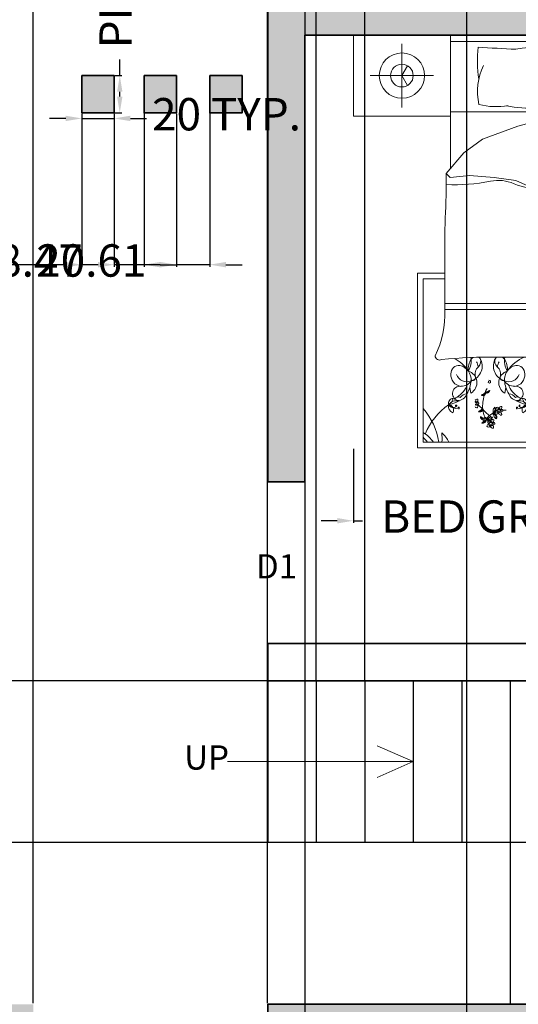
# Model space of a CAD drawing. Units: centimetres. Extents: x 2137 to 3697, y 183 to 2094.
# Tile 5 of 8: x 3031 to 3339, y 600 to 1208. Entities that reach past the tile are written whole.
import ezdxf

# ---------------------------------------------------------------- set-up
doc = ezdxf.new("R2010")
doc.units = ezdxf.units.CM
for name, color, linetype, lineweight in [('A-ANNO-DIMS', 2, 'Continuous', 18), ('A-ANNO-SYMB', 7, 'Continuous', 18), ('A-ANNO-TEXT', 7, 'Continuous', 18), ('A-COLS', 7, 'Continuous', 35), ('A-COLS-PATT', 52, 'Continuous', 13), ('A-FLOR-STRS', 7, 'Continuous', 25), ('A-FURN', 8, 'Continuous', 18), ('A-WALL', 7, 'Continuous', 35), ('A-WALL-PATT', 52, 'Continuous', 13)]:
    doc.layers.add(name, color=color, linetype=linetype, lineweight=lineweight)
doc.styles.get("Standard").update_dxf_attribs({"font": 'arial.ttf'})
doc.dimstyles.new('ISO-25', dxfattribs={"dimtxt": 20, "dimasz": 10, "dimexe": 1.25, "dimexo": 0.625, "dimtad": 0, "dimtxsty": 'Standard', "dimcen": 2.5, "dimadec": 0, "dimazin": 0, "dimtfac": 1, "dimtmove": 0, "dimatfit": 3, "dimfxl": 1, "dimarcsym": 0})

# ---------------------------------------------------------------- blocks, each defined once
blk = doc.blocks.new('BED')
for p, q in [((2442.52, 2474.71), (2742.52, 2474.71)), ((2502.52, 2474.71), (2502.52, 2392.37)), ((2682.52, 2470.86), (2502.52, 2470.86)), ((2472.52, 2430.11), (2472.52, 2469.31)), ((2712.52, 2430.11), (2712.52, 2469.31)), ((2492.12, 2449.71), (2452.92, 2449.71)), ((2692.92, 2449.71), (2732.12, 2449.71)), ((2502.52, 2427.3), (2682.52, 2427.3)), ((2544.19, 2418.38), (2576.9, 2427.3)), ((2584.93, 2427.3), (2568.49, 2404.42)), ((2522.31, 2410.49), (2544.19, 2418.38)), ((2510.77, 2401.99), (2522.31, 2410.49)), ((2681.6, 2411.76), (2572.66, 2410.22)), ((2681.71, 2414.84), (2574.9, 2413.34)), ((2568.49, 2404.42), (2561.81, 2386.81)), ((2499.83, 2389.24), (2510.77, 2401.99)), ((2681.46, 2399.23), (2566.35, 2398.76)), ((2681.44, 2402.31), (2567.52, 2401.86)), ((2502.26, 2386.81), (2499.83, 2389.24)), ((2514.41, 2388.02), (2502.26, 2386.81)), ((2529.61, 2386.81), (2514.41, 2388.02)), ((2542.97, 2384.99), (2529.61, 2386.81)), ((2561.81, 2386.81), (2560.59, 2378.91)), ((2550.87, 2381.34), (2542.97, 2384.99)), ((2560.59, 2378.91), (2550.87, 2381.34)), ((2482.11, 2327.65), (2499.08, 2327.65)), ((2482.11, 2219.58), (2482.11, 2327.65)), ((2684.19, 2327.65), (2700.83, 2327.65)), ((2700.83, 2327.65), (2700.83, 2219.58)), ((2499.08, 2324.17), (2485.59, 2324.17)), ((2485.59, 2324.17), (2485.59, 2223.06)), ((2697.35, 2324.17), (2684.13, 2324.17)), ((2697.35, 2223.06), (2697.35, 2324.17)), ((2683.88, 2308.94), (2499.06, 2308.94)), ((2684.17, 2305.2), (2499.06, 2305.2)), ((2653.42, 2275.73), (2531.62, 2275.73)), ((2515.15, 2253.47), (2514.49, 2256.86)), ((2536.12, 2253.47), (2536.78, 2256.86)), ((2646.82, 2253.47), (2646.16, 2256.86)), ((2667.79, 2253.47), (2668.45, 2256.86)), ((2485.59, 2223.06), (2697.35, 2223.06)), ((2700.83, 2219.58), (2482.11, 2219.58))]:
    blk.add_line(p, q)
for points in [[(2502.52, 2424.71), (2442.52, 2424.71), (2442.52, 2474.71)], [(2682.52, 2474.71), (2682.52, 2424.71), (2742.52, 2424.71), (2742.52, 2474.71)], [(2472.52, 2449.71), (2476.02, 2455.77)], [(2712.52, 2449.71), (2709.02, 2455.77)], [(2472.52, 2449.71), (2476.02, 2443.65)], [(2712.52, 2449.71), (2709.02, 2443.65)]]:
    blk.add_lwpolyline(points)
for points in [[(2519.75, 2467.23, 0.074897), (2520.11, 2447.64, -0.472817)], [(2591.11, 2446.54, 0.14099), (2591.71, 2466.53, 0.235245)], [(2603.92, 2446.54, -0.14099), (2603.32, 2466.53, -0.235245)], [(2665.29, 2467.23, -0.074897), (2664.92, 2447.64, 0.472817)], [(2499.2, 2361.77, 0.001242), (2499.06, 2304.85, -0.127202), (2493.05, 2276.48)], [(2683.8, 2311.3, 0.056112), (2685.97, 2294.79, 0.095341), (2690.19, 2278.9)]]:
    blk.add_lwpolyline(points, format="xyb")
for centre, radius in [((2472.52, 2449.71), 14), ((2712.52, 2449.71), 14), ((2472.52, 2449.71), 7), ((2712.52, 2449.71), 7), ((2532.49, 2242.6), 0.764), ((2650.46, 2242.6), 0.764), ((2527.49, 2234.55), 0.764), ((2655.45, 2234.55), 0.764)]:
    blk.add_circle(centre, radius)
for centre, radius, start, end in [((2685.11, 5322.24), 2859.79, 266.68521, 267.14978), ((2560.85, 2358.67), 108.8, 82.21958, 99.49698), ((2583.83, 2413.66), 53.46, 81.52493, 103.95996), ((2607.44, 2452.27), 14.84, 63.34374, 106.10256), ((2629.68, 2414.74), 52.74, 76.34271, 101.1841), ((2499.93, 5322.24), 2859.79, 272.85022, 273.31479), ((2557.97, 2439.77), 38.67, 155.1316, 191.75834), ((2627.07, 2439.77), 38.67, 348.24166, 24.8684), ((2555.75, 2436.51), 36.76, 354.01289, 15.82928), ((2639.29, 2436.51), 36.76, 164.17072, 185.98711), ((2530.45, 2470.74), 40.2, 255.10393, 281.03689), ((2551.61, 2499.32), 69.73, 258.03974, 289.26152), ((2579.84, 2484.1), 52.9, 259.86169, 283.62376), ((2609.45, 2447.1), 15.9, 245.01826, 288.54073), ((2637.23, 2467.78), 38.19, 243.87611, 286.17464), ((2654.58, 2470.74), 40.2, 258.96311, 284.89607), ((3220.32, 2390.64), 539.05, 176.09997, 180.92818), ((2224.76, 2381.78), 275.17, 355.82941, 1.55305), ((2504.97, 2495.47), 113.22, 267.45188, 281.3392), ((2532.03, 2360.52), 24.42, 66.26158, 101.3392), ((2581.42, 2492.28), 116.34, 250.11942, 259.33829), ((3384.42, 2371.04), 703.17, 179.11454, 184.87351), ((2559.91, 2378.67), 0.724, 268.86235, 19.75363), ((2495.81, 2276.67), 2.77, 183.97998, 297.34124), ((2687.92, 2277.37), 2.73, 246.52186, 33.82642), ((2528.04, 1963.45), 312.3, 89.34325, 95.68869), ((2507.86, 2265.5), 5.07, 84.48557, 181.05378), ((2494.64, 2254.6), 22.71, 33.66712, 63.29966), ((2506.31, 2261.76), 9.02, 355.29334, 76.921), ((2525.07, 2268.11), 11.57, 145.78505, 184.73037), ((2502.97, 2273.51), 12.43, 328.82178, 9.15542), ((2518.36, 2272.41), 3.61, 120.0293, 142.32497), ((2512.59, 2270.28), 9.56, 289.28218, 29.1751), ((2511.15, 2268.55), 8.62, 7.43599, 29.91487), ((2516.83, 2273.13), 4.49, 311.56531, 23.83541), ((2518.36, 2272.41), 3.61, 44.45169, 63.55801), ((2538.68, 2270.28), 9.56, 150.8249, 250.71782), ((2534.44, 2273.13), 4.49, 156.16459, 228.43469), ((2532.91, 2272.41), 3.61, 113.22901, 135.54831), ((2540.13, 2268.55), 8.62, 150.08513, 172.56401), ((2532.91, 2272.41), 3.61, 37.67503, 66.71436), ((2526.21, 2268.11), 11.57, 355.26963, 34.21495), ((2548.31, 2273.51), 12.43, 169.71335, 211.17822), ((2544.97, 2261.76), 9.02, 103.079, 184.70666), ((2556.64, 2254.6), 22.71, 111.49413, 146.33288), ((2543.41, 2265.5), 5.07, 358.94622, 95.51443), ((2639.53, 2265.5), 5.07, 84.48557, 181.05378), ((2626.3, 2254.6), 22.71, 33.66712, 68.50587), ((2637.98, 2261.76), 9.02, 355.29334, 76.921), ((2656.73, 2268.11), 11.57, 145.78505, 184.73037), ((2634.63, 2273.51), 12.43, 328.82178, 10.28665), ((2650.03, 2272.41), 3.61, 113.28564, 142.32497), ((2644.26, 2270.28), 9.56, 289.28218, 29.1751), ((2642.81, 2268.55), 8.62, 7.43599, 29.91487), ((2650.03, 2272.41), 3.61, 44.45169, 66.71436), ((2648.5, 2273.13), 4.49, 311.56531, 23.83541), ((2662.61, 1983.95), 291.92, 85.24024, 91.80351), ((2670.35, 2270.28), 9.56, 150.8249, 250.71782), ((2666.11, 2273.13), 4.49, 156.16459, 228.43469), ((2664.58, 2272.41), 3.61, 106.63434, 135.54831), ((2671.79, 2268.55), 8.62, 150.08513, 172.56401), ((2664.58, 2272.41), 3.61, 37.67503, 72.58143), ((2657.87, 2268.11), 11.57, 355.26963, 34.21495), ((2679.98, 2273.51), 12.43, 169.24899, 211.17822), ((2676.63, 2261.76), 9.02, 103.079, 184.70666), ((2688.3, 2254.6), 22.71, 113.64533, 146.33288), ((2675.08, 2265.5), 5.07, 358.94622, 95.51443), ((2509.94, 2264.78), 7.17, 174.94485, 262.88575), ((2512.76, 2267.5), 6.96, 201.58187, 291.42215), ((2511.44, 2259.94), 7.46, 299.90854, 73.1337), ((2523.89, 2265.16), 6.15, 131.56531, 195.14713), ((2527.38, 2265.16), 6.15, 344.85287, 48.43469), ((2539.84, 2259.94), 7.46, 106.8663, 240.09146), ((2538.52, 2267.5), 6.96, 248.57785, 338.41813), ((2541.33, 2264.78), 7.17, 277.11425, 5.05515), ((2641.61, 2264.78), 7.17, 174.94485, 262.88575), ((2644.43, 2267.5), 6.96, 201.58187, 291.42215), ((2643.1, 2259.94), 7.46, 299.90854, 73.1337), ((2655.56, 2265.16), 6.15, 131.56531, 195.14713), ((2659.05, 2265.16), 6.15, 344.85287, 48.43469), ((2671.51, 2259.94), 7.46, 106.8663, 240.09146), ((2670.18, 2267.5), 6.96, 248.57785, 338.41813), ((2673, 2264.78), 7.17, 277.11425, 5.05515), ((2499.37, 2263.14), 14.16, 301.26137, 341.7045), ((2508.7, 2266.37), 8.71, 272.3591, 324.04014), ((2499.23, 2262), 16.1, 326.28828, 356.5076), ((2525.07, 2268.11), 11.57, 212.70113, 216.34448), ((2516.16, 2263.07), 1.86, 257.30406, 15.14713), ((2526.5, 2260.25), 0.578, 102.70507, 280.43845), ((2526.43, 2260.6), 0.94, 280.43845, 100.41356), ((2535.12, 2263.07), 1.86, 164.85287, 282.69594), ((2526.21, 2268.11), 11.57, 323.65552, 327.29887), ((2542.58, 2266.37), 8.71, 215.95986, 267.6409), ((2552.04, 2262), 16.1, 183.4924, 213.71172), ((2551.91, 2263.14), 14.16, 198.2955, 238.73863), ((2594.92, 2255.93), 3.25, 63.02737, 163.80375), ((2591.63, 2263.52), 6.69, 271.45846, 315.37266), ((2598.02, 2255.93), 3.25, 16.19625, 116.97263), ((2601.31, 2263.52), 6.69, 224.62734, 268.54154), ((2631.03, 2263.14), 14.16, 301.26137, 341.7045), ((2640.36, 2266.37), 8.71, 272.3591, 324.04014), ((2630.9, 2262), 16.1, 326.28828, 356.5076), ((2656.73, 2268.11), 11.57, 212.70113, 216.34448), ((2647.82, 2263.07), 1.86, 257.30406, 15.14713), ((2656.51, 2260.6), 0.94, 79.58644, 259.56155), ((2656.44, 2260.25), 0.578, 259.56155, 77.29493), ((2666.78, 2263.07), 1.86, 164.85287, 282.69594), ((2657.87, 2268.11), 11.57, 323.65552, 327.29887), ((2674.25, 2266.37), 8.71, 215.95986, 267.6409), ((2683.71, 2262), 16.1, 183.4924, 213.71172), ((2683.58, 2263.14), 14.16, 198.2955, 238.73863), ((2508.29, 2253.23), 4.5, 80.26398, 250.86884), ((2507.21, 2254.58), 5.62, 265.96902, 344.3045), ((2513.27, 2247.11), 5.99, 96.1662, 141.58255), ((2523.19, 2251.31), 1.58, 101.32561, 154.46214), ((2520.92, 2256.65), 4.74, 280.25878, 300.65599), ((2522.01, 2260.45), 8.46, 268.32639, 277.13024), ((2547.29, 2245.15), 24.85, 163.58418, 183.82768), ((2519.89, 2256.64), 4.82, 308.21012, 316.30712), ((2522.85, 2253.47), 1.44, 278.34322, 4.28685), ((2522.06, 2254.74), 2.51, 300.65599, 332.63414), ((2523.94, 2253.08), 0.611, 55.76575, 157.44165), ((2547.29, 2245.15), 24.85, 153.0032, 159.89408), ((2524.9, 2253.65), 0.611, 84.37838, 186.05427), ((2524.32, 2256.1), 2.51, 269.18588, 301.16403), ((2525.06, 2254.8), 1.44, 237.53317, 323.47681), ((2523.67, 2258.9), 4.82, 285.51291, 293.60991), ((2526.81, 2253.48), 1.58, 87.35788, 140.49441), ((2523.17, 2258), 4.74, 301.16403, 321.56124), ((2519.31, 2258.83), 8.46, 324.68979, 333.49364), ((2538.01, 2247.11), 5.99, 38.41745, 83.8338), ((2544.06, 2254.58), 5.62, 195.6955, 274.03098), ((2542.98, 2253.23), 4.5, 289.13116, 99.73602), ((2594.85, 2217.78), 39.18, 94.46233, 172.25504), ((2595.02, 2253.92), 4.34, 137.78732, 219.11446), ((2590.09, 2254.05), 3.27, 298.5391, 58.36268), ((2594.35, 2251.19), 6.19, 45.54113, 114.31008), ((2600, 2282.98), 27.41, 252.59304, 267.25817), ((2595, 2256.71), 3.2, 177.75849, 283.85198), ((2601.17, 2260.05), 9.91, 198.91595, 238.01098), ((2598.59, 2251.19), 6.19, 65.68992, 134.45887), ((2592.94, 2282.98), 27.41, 272.74183, 287.40696), ((2595.67, 2254.01), 0.424, 283.85198, 219.92454), ((2596.18, 2252.06), 0.487, 238.01098, 71.55918), ((2596.26, 2252.29), 0.236, 71.55918, 188.01668), ((2596.76, 2252.06), 0.487, 108.44082, 301.98902), ((2596.68, 2252.29), 0.236, 351.98332, 108.44082), ((2597.23, 2254.17), 0.255, 320.19092, 256.02088), ((2591.77, 2260.05), 9.91, 301.98902, 341.08405), ((2597.94, 2256.71), 3.2, 256.14802, 2.24151), ((2602.86, 2254.05), 3.27, 121.63732, 241.4609), ((2597.92, 2253.92), 4.34, 320.88554, 42.21268), ((2596.83, 2226.82), 30.32, 352.86355, 81.81966), ((2639.96, 2253.23), 4.5, 80.26398, 250.86884), ((2638.88, 2254.58), 5.62, 265.96902, 344.3045), ((2644.93, 2247.11), 5.99, 96.1662, 141.58255), ((2656.13, 2253.48), 1.58, 39.50559, 92.64212), ((2659.77, 2258), 4.74, 218.43876, 238.83597), ((2663.63, 2258.83), 8.46, 206.50636, 215.31021), ((2657.88, 2254.8), 1.44, 216.52319, 302.46683), ((2658.62, 2256.1), 2.51, 238.83597, 270.81412), ((2659.27, 2258.9), 4.82, 246.39009, 254.48709), ((2635.65, 2245.15), 24.85, 20.10592, 26.9968), ((2658.05, 2253.65), 0.611, 353.94573, 95.62162), ((2659, 2253.08), 0.611, 22.55835, 124.23425), ((2660.09, 2253.47), 1.44, 175.71315, 261.65678), ((2660.89, 2254.74), 2.51, 207.36586, 239.34401), ((2635.65, 2245.15), 24.85, 356.17232, 16.41582), ((2663.05, 2256.64), 4.82, 223.69288, 231.78988), ((2662.02, 2256.65), 4.74, 239.34401, 259.74122), ((2660.93, 2260.45), 8.46, 262.86976, 271.67361), ((2659.76, 2251.31), 1.58, 25.53786, 78.67439), ((2675.73, 2254.58), 5.62, 195.6955, 274.03098), ((2669.67, 2247.11), 5.99, 38.41745, 83.8338), ((2674.65, 2253.23), 4.5, 289.13116, 99.73602), ((2523.45, 2213.9), 39.18, 124.38655, 158.59079), ((2505.57, 2245.31), 4.34, 167.71153, 249.03868), ((2504.48, 2247), 3.25, 92.95159, 193.72796), ((2497.84, 2251.95), 6.69, 301.38267, 345.29688), ((2506.35, 2242.61), 6.19, 75.46535, 144.23429), ((2495.38, 2272.99), 27.41, 282.51726, 297.18239), ((2501.23, 2242.96), 3.27, 328.46331, 88.28689), ((2507.84, 2253.69), 9.91, 228.84017, 267.9352), ((2504.16, 2247.72), 3.2, 207.6827, 313.77619), ((2507.37, 2248.35), 2.76, 63.97555, 143.26805), ((2506.09, 2245.71), 0.424, 313.77619, 249.71835), ((2518.73, 2248.32), 1.27, 101.56373, 142.6358), ((2517.68, 2247.14), 0.764, 273.27684, 86.72316), ((2518.57, 2247.86), 0.73, 91.10805, 181.86747), ((2520.08, 2247.41), 2.32, 203.42757, 227.61037), ((2519.34, 2246.4), 1.58, 80.3487, 133.65382), ((2519.06, 2247.7), 1.25, 229.78892, 317.67915), ((2517.71, 2249.32), 1.84, 288.72627, 352.50315), ((2517.65, 2245.06), 1.78, 355.05304, 68.36176), ((2519.04, 2244.75), 2.5, 83.08516, 105.71709), ((2518.96, 2249.23), 0.59, 345.23556, 144.9248), ((2501.72, 2224.01), 28.48, 43.15413, 52.0459), ((2519.5, 2247.3), 0.658, 317.67915, 80.3487), ((2543.91, 2248.35), 2.76, 36.73195, 116.02445), ((2544.93, 2242.61), 6.19, 35.76571, 104.53465), ((2555.89, 2272.99), 27.41, 242.81761, 257.48274), ((2543.43, 2253.69), 9.91, 272.0648, 311.15983), ((2547.11, 2247.72), 3.2, 226.22381, 332.3173), ((2545.24, 2245.88), 0.255, 290.26671, 226.22708), ((2550.05, 2242.96), 3.27, 91.71311, 211.53669), ((2546.8, 2247), 3.25, 346.27204, 87.04841), ((2553.44, 2251.95), 6.69, 194.70312, 238.61733), ((2545.71, 2245.31), 4.34, 290.96132, 12.28847), ((2527.83, 2213.9), 39.18, 21.40921, 55.61345), ((2655.12, 2213.9), 39.18, 124.38655, 158.59079), ((2637.23, 2245.31), 4.34, 167.71153, 249.03868), ((2636.14, 2247), 3.25, 92.95159, 193.72796), ((2629.51, 2251.95), 6.69, 301.38267, 345.29688), ((2638.02, 2242.61), 6.19, 75.46535, 144.23429), ((2627.05, 2272.99), 27.41, 282.51726, 297.18239), ((2635.83, 2247.72), 3.2, 207.6827, 313.77619), ((2639.51, 2253.69), 9.91, 228.84017, 267.9352), ((2632.89, 2242.96), 3.27, 328.46331, 88.28689), ((2639.03, 2248.35), 2.76, 63.97555, 143.26805), ((2637.75, 2245.71), 0.424, 313.77619, 249.71835), ((2681.22, 2224.01), 28.48, 127.9541, 136.84587), ((2663.45, 2247.3), 0.658, 99.6513, 222.32085), ((2663.88, 2247.7), 1.25, 222.32085, 310.21108), ((2663.6, 2246.4), 1.58, 46.34618, 99.6513), ((2663.98, 2249.23), 0.59, 35.0752, 194.76444), ((2665.23, 2249.32), 1.84, 187.49685, 251.27373), ((2665.29, 2245.06), 1.78, 111.63824, 184.94696), ((2663.9, 2244.75), 2.5, 74.28291, 96.91484), ((2664.38, 2247.86), 0.73, 358.13253, 88.89195), ((2662.86, 2247.41), 2.32, 312.38963, 336.57243), ((2664.21, 2248.32), 1.27, 37.3642, 78.43627), ((2665.27, 2247.14), 0.764, 93.27684, 266.72316), ((2675.58, 2248.35), 2.76, 36.73195, 116.02445), ((2676.59, 2242.61), 6.19, 35.76571, 104.53465), ((2687.56, 2272.99), 27.41, 242.81761, 257.48274), ((2675.1, 2253.69), 9.91, 272.0648, 311.15983), ((2678.78, 2247.72), 3.2, 226.22381, 332.3173), ((2676.9, 2245.88), 0.255, 290.26671, 226.22708), ((2681.72, 2242.96), 3.27, 91.71311, 211.53669), ((2685.1, 2251.95), 6.69, 194.70312, 238.61733), ((2678.46, 2247), 3.25, 346.27204, 87.04841), ((2677.37, 2245.31), 4.34, 290.96132, 12.28847), ((2659.49, 2213.9), 39.18, 21.40921, 55.61345), ((2456.43, 2217.78), 39.18, 7.74496, 41.8856), ((2507.46, 2244.52), 0.236, 101.4834, 217.94089), ((2507.5, 2244.28), 0.487, 267.9352, 101.4834), ((2518.72, 2245.73), 1.26, 217.76209, 259.04026), ((2518.83, 2244.95), 0.586, 232.47371, 355.05304), ((2521.4, 2241.21), 1.58, 101.32561, 154.46214), ((2519.13, 2246.56), 4.74, 280.25878, 300.65599), ((2520.22, 2250.35), 8.46, 268.32639, 277.13024), ((2518.11, 2246.55), 4.82, 308.21012, 316.30712), ((2521.07, 2243.38), 1.44, 278.34322, 4.28685), ((2520.27, 2244.64), 2.51, 300.65599, 332.63414), ((2522.16, 2242.98), 0.611, 55.76575, 157.44165), ((2534.91, 2244.52), 12.46, 184.75602, 209.20408), ((2552.85, 2271.04), 40.99, 222.24124, 232.17444), ((2536.2, 2227.98), 14.94, 120.54402, 139.81798), ((2528.5, 2242.96), 2.12, 272.84988, 356.12261), ((2526.64, 2243.74), 3.48, 304.53686, 16.36991), ((2527, 2242.14), 2.05, 321.76073, 7.92519), ((2527.43, 2239.19), 2.05, 8.72271, 54.88717), ((2527.54, 2237.55), 3.48, 0.278, 72.11105), ((2531.47, 2242.76), 2.46, 127.31045, 187.92519), ((2529.1, 2238.83), 2.12, 20.5253, 88.5375), ((2528.09, 2243.04), 2.53, 355.01064, 41.65801), ((2530.88, 2241.17), 0.757, 148.0499, 225.62681), ((2536.2, 2227.98), 14.94, 113.05007, 113.84774), ((2532.28, 2240.29), 2.41, 104.75581, 148.0499), ((2530.93, 2242.02), 1.51, 247.40857, 351.43859), ((2531.64, 2243.66), 1.04, 126.10456, 271.42811), ((2528.73, 2238.64), 2.53, 334.9899, 21.63727), ((2531.53, 2243.95), 0.749, 353.75256, 131.70535), ((2531.35, 2241.96), 0.506, 262.90601, 7.13198), ((2530.82, 2243.06), 1.05, 0.06451, 61.15075), ((2531.07, 2243.95), 1.2, 311.84125, 355.78771), ((2533.54, 2243.78), 1.27, 101.56373, 176.36503), ((2533.53, 2241.19), 1.26, 151.21959, 259.04026), ((2533.38, 2243.32), 0.73, 91.10805, 181.86747), ((2534.89, 2242.87), 2.32, 203.42757, 227.61037), ((2534.15, 2241.86), 1.58, 80.3487, 133.65382), ((2533.87, 2243.16), 1.25, 229.78892, 317.67915), ((2532.52, 2244.78), 1.84, 288.72627, 352.50315), ((2532.46, 2240.51), 1.78, 355.05304, 68.36176), ((2533.85, 2240.21), 2.5, 83.08516, 105.71709), ((2533.77, 2244.69), 0.59, 345.23556, 144.9248), ((2533.64, 2240.41), 0.586, 232.47371, 355.05304), ((2534.31, 2242.76), 0.658, 317.67915, 80.3487), ((2536.2, 2227.98), 14.94, 87.10709, 94.75853), ((2543.77, 2244.28), 0.487, 78.5166, 272.0648), ((2543.82, 2244.52), 0.236, 322.05911, 78.5166), ((2639.12, 2244.52), 0.236, 101.4834, 217.94089), ((2639.17, 2244.28), 0.487, 267.9352, 101.4834), ((2646.75, 2227.98), 14.94, 85.24147, 92.89291), ((2648.64, 2242.76), 0.658, 99.6513, 222.32085), ((2649.07, 2243.16), 1.25, 222.32085, 310.21108), ((2648.79, 2241.86), 1.58, 46.34618, 99.6513), ((2649.17, 2244.69), 0.59, 35.0752, 194.76444), ((2650.42, 2244.78), 1.84, 187.49685, 251.27373), ((2650.48, 2240.51), 1.78, 111.63824, 184.94696), ((2649.3, 2240.41), 0.586, 184.94696, 307.52629), ((2649.09, 2240.21), 2.5, 74.28291, 96.91484), ((2649.56, 2243.32), 0.73, 358.13253, 88.89195), ((2648.05, 2242.87), 2.32, 312.38963, 336.57243), ((2649.4, 2243.78), 1.27, 3.63497, 78.43627), ((2649.41, 2241.19), 1.26, 280.95974, 28.78041), ((2652.01, 2242.02), 1.51, 188.56141, 292.59143), ((2651.41, 2243.95), 0.749, 48.29465, 186.24744), ((2651.87, 2243.95), 1.2, 184.21229, 228.15875), ((2652.12, 2243.06), 1.05, 118.84925, 179.93549), ((2651.59, 2241.96), 0.506, 172.86802, 277.09399), ((2651.3, 2243.66), 1.04, 268.57189, 53.89544), ((2650.66, 2240.29), 2.41, 31.9501, 75.24419), ((2654.21, 2238.64), 2.53, 158.36273, 205.0101), ((2653.84, 2238.83), 2.12, 91.4625, 159.4747), ((2655.4, 2237.55), 3.48, 107.88895, 179.722), ((2654.85, 2243.04), 2.53, 138.34199, 184.98936), ((2654.44, 2242.96), 2.12, 183.87739, 267.15012), ((2652.06, 2241.17), 0.757, 314.37319, 31.9501), ((2646.75, 2227.98), 14.94, 66.15226, 66.94993), ((2656.3, 2243.74), 3.48, 163.63009, 235.46314), ((2651.47, 2242.76), 2.46, 352.07481, 52.68955), ((2655.51, 2239.19), 2.05, 125.11283, 171.27729), ((2655.94, 2242.14), 2.05, 172.07481, 218.23927), ((2646.75, 2227.98), 14.94, 40.18202, 59.45598), ((2630.09, 2271.04), 40.99, 307.82556, 317.75876), ((2648.03, 2244.52), 12.46, 330.79592, 355.24398), ((2660.78, 2242.98), 0.611, 22.55835, 124.23425), ((2661.88, 2243.38), 1.44, 175.71315, 261.65678), ((2662.67, 2244.64), 2.51, 207.36586, 239.34401), ((2664.83, 2246.55), 4.82, 223.69288, 231.78988), ((2663.81, 2246.56), 4.74, 239.34401, 259.74122), ((2662.72, 2250.35), 8.46, 262.86976, 271.67361), ((2661.54, 2241.21), 1.58, 25.53786, 78.67439), ((2664.11, 2244.95), 0.586, 184.94696, 307.52629), ((2664.23, 2245.73), 1.26, 280.95974, 322.23791), ((2675.44, 2244.28), 0.487, 78.5166, 272.0648), ((2675.49, 2244.52), 0.236, 322.05911, 78.5166), ((2726.52, 2217.78), 39.18, 138.1144, 172.25504), ((2521.93, 2238.45), 0.853, 146.86359, 236.90213), ((2533.96, 2257.24), 22.32, 235.1882, 238.88441), ((2523.39, 2239.69), 2.31, 199.47987, 267.68284), ((2523.14, 2238.82), 1.99, 212.81548, 277.39917), ((2521.98, 2237.49), 2.31, 266.97007, 338.29129), ((2509.81, 2253.97), 22.32, 302.6784, 306.37461), ((2522.56, 2235.66), 0.853, 214.3538, 304.39233), ((2522.88, 2238.89), 0.883, 238.88441, 314.26458), ((2522.69, 2236.91), 1.99, 280.30568, 17.1958), ((2522.52, 2236.71), 0.883, 306.37461, 21.75478), ((2523.96, 2237.28), 0.666, 19.36054, 201.75478), ((2523.96, 2237.78), 0.666, 311.87034, 134.26458), ((2536.49, 2231.71), 13.31, 153.78194, 158.29129), ((2525.9, 2240.8), 3.48, 247.23048, 319.06353), ((2524.75, 2239.63), 2.05, 264.45436, 310.61881), ((2534.91, 2244.52), 12.46, 214.00334, 222.49171), ((2526.25, 2238.81), 2.12, 218.32082, 298.81623), ((2525.88, 2233.11), 0.757, 148.0499, 225.62681), ((2527.28, 2232.24), 2.41, 104.75581, 148.0499), ((2525.93, 2233.96), 1.51, 247.40857, 351.43859), ((2526.65, 2235.61), 1.04, 126.10456, 271.42811), ((2526.53, 2235.89), 0.749, 353.75256, 131.70535), ((2527.69, 2236.2), 2.46, 70.00407, 130.61881), ((2526.36, 2233.9), 0.506, 262.90601, 7.13198), ((2525.83, 2235), 1.05, 0.06451, 61.15075), ((2526.08, 2235.9), 1.2, 311.84125, 355.78771), ((2526.09, 2239.2), 2.53, 297.70426, 344.35163), ((2528.55, 2235.73), 1.27, 101.56373, 176.36503), ((2528.53, 2233.13), 1.26, 151.21959, 259.04026), ((2528.38, 2235.27), 0.73, 91.10805, 181.86747), ((2529.89, 2234.81), 2.32, 203.42757, 227.61037), ((2529.15, 2233.8), 1.58, 80.3487, 133.65382), ((2528.87, 2235.11), 1.25, 229.78892, 317.67915), ((2527.52, 2236.73), 1.84, 288.72627, 352.50315), ((2527.46, 2232.46), 1.78, 355.05304, 68.36176), ((2528.85, 2232.16), 2.5, 83.08516, 105.71709), ((2528.77, 2236.64), 0.59, 345.23556, 144.9248), ((2529.31, 2234.71), 0.658, 317.67915, 80.3487), ((2531.89, 2239.88), 2.46, 188.72271, 249.33746), ((2591.85, 2196.79), 39.18, 94.46233, 117.4146), ((2592.02, 2232.93), 4.34, 137.78732, 219.11446), ((2587.09, 2233.07), 3.27, 298.5391, 58.36268), ((2591.92, 2234.94), 3.25, 63.02737, 163.80375), ((2588.63, 2242.54), 6.69, 271.45846, 315.37266), ((2591.35, 2230.21), 6.19, 45.54113, 114.31008), ((2598.17, 2239.06), 9.91, 198.91595, 238.01098), ((2597, 2262), 27.41, 252.59304, 267.25817), ((2592, 2235.73), 3.2, 177.75849, 283.85198), ((2601.59, 2230.21), 6.19, 65.68992, 134.45887), ((2595.94, 2262), 27.41, 272.74183, 287.40696), ((2601.02, 2234.94), 3.25, 16.19625, 116.97263), ((2604.31, 2242.54), 6.69, 224.62734, 268.54154), ((2594.77, 2239.06), 9.91, 301.98902, 341.08405), ((2600.94, 2235.73), 3.2, 256.14802, 2.24151), ((2605.86, 2233.07), 3.27, 121.63732, 241.4609), ((2600.92, 2232.93), 4.34, 320.88554, 42.21268), ((2601.09, 2196.79), 39.18, 62.5854, 85.53767), ((2651.05, 2239.88), 2.46, 290.66254, 351.27729), ((2653.63, 2234.71), 0.658, 99.6513, 222.32085), ((2654.07, 2235.11), 1.25, 222.32085, 310.21108), ((2653.79, 2233.8), 1.58, 46.34618, 99.6513), ((2654.17, 2236.64), 0.59, 35.0752, 194.76444), ((2655.42, 2236.73), 1.84, 187.49685, 251.27373), ((2655.48, 2232.46), 1.78, 111.63824, 184.94696), ((2654.09, 2232.16), 2.5, 74.28291, 96.91484), ((2655.26, 2236.2), 2.46, 49.38119, 109.99593), ((2657.04, 2240.8), 3.48, 220.93647, 292.76952), ((2656.85, 2239.2), 2.53, 195.64837, 242.29574), ((2654.56, 2235.27), 0.73, 358.13253, 88.89195), ((2653.05, 2234.81), 2.32, 312.38963, 336.57243), ((2654.4, 2235.73), 1.27, 3.63497, 78.43627), ((2654.41, 2233.13), 1.26, 280.95974, 28.78041), ((2657.01, 2233.96), 1.51, 188.56141, 292.59143), ((2656.41, 2235.89), 0.749, 48.29465, 186.24744), ((2656.69, 2238.81), 2.12, 241.18377, 321.67918), ((2656.87, 2235.9), 1.2, 184.21229, 228.15875), ((2657.12, 2235), 1.05, 118.84925, 179.93549), ((2656.58, 2233.9), 0.506, 172.86802, 277.09399), ((2656.3, 2235.61), 1.04, 268.57189, 53.89544), ((2655.66, 2232.24), 2.41, 31.9501, 75.24419), ((2658.19, 2239.63), 2.05, 229.38119, 275.54564), ((2648.03, 2244.52), 12.46, 317.50829, 325.99666), ((2657.06, 2233.11), 0.757, 314.37319, 31.9501), ((2660.25, 2236.91), 1.99, 162.8042, 259.69432), ((2658.98, 2237.78), 0.666, 45.73542, 228.12966), ((2658.98, 2237.28), 0.666, 338.24522, 160.63946), ((2646.45, 2231.71), 13.31, 21.70871, 26.21806), ((2660.96, 2237.49), 2.31, 201.70871, 273.02993), ((2660.06, 2238.89), 0.883, 225.73542, 301.11559), ((2660.42, 2236.71), 0.883, 158.24522, 233.62539), ((2659.81, 2238.82), 1.99, 262.60083, 327.18452), ((2659.55, 2239.69), 2.31, 272.31716, 340.52013), ((2673.14, 2253.97), 22.32, 233.62539, 237.3216), ((2660.38, 2235.66), 0.853, 235.60767, 325.6462), ((2648.98, 2257.24), 22.32, 301.11559, 304.8118), ((2661.01, 2238.45), 0.853, 303.09787, 33.13641), ((2476.08, 2212.53), 19.09, 33.46172, 60.11157), ((2486.77, 2216.95), 15.93, 22.55474, 48.95456), ((2443.14, 2225.51), 54.2, 357.40811, 3.65191), ((2528.65, 2232.36), 0.586, 232.47371, 355.05304), ((2564.51, 2216.95), 15.93, 131.04544, 157.44526), ((2608.14, 2225.51), 54.2, 176.34809, 182.59189), ((2575.2, 2212.53), 19.09, 91.27197, 146.53828), ((2582.06, 2208.97), 23.79, 107.85038, 143.69643), ((2594.57, 2202.28), 35.39, 124.01234, 144.05304), ((2592.67, 2233.03), 0.424, 283.85198, 219.92454), ((2593.18, 2231.07), 0.487, 238.01098, 71.55918), ((2593.26, 2231.31), 0.236, 71.55918, 188.01668), ((2599.76, 2231.07), 0.487, 108.44082, 301.98902), ((2599.68, 2231.31), 0.236, 351.98332, 108.44082), ((2600.23, 2233.19), 0.255, 320.19092, 256.02088), ((2600.75, 2229.59), 17.54, 338.11703, 6.61954), ((2616.84, 2224.71), 7.03, 346.38982, 79.07385), ((2611.55, 2225.68), 8.89, 342.86088, 41.90487), ((2574.8, 2225.51), 54.2, 357.40811, 3.65191), ((2618.44, 2216.95), 15.93, 22.55474, 48.95456), ((2654.29, 2232.36), 0.586, 184.94696, 307.52629), ((2696.17, 2216.95), 15.93, 131.04544, 157.44526), ((2739.8, 2225.51), 54.2, 176.34809, 182.59189), ((2706.86, 2212.53), 19.09, 119.88843, 146.53828), ((2469.21, 2208.97), 23.79, 36.30357, 46.48142), ((2580.89, 2202.46), 21.54, 73.54311, 107.0202), ((2589.43, 2191.36), 31.85, 94.37872, 95.63574), ((2606.21, 2169.53), 56.92, 109.72171, 109.90284), ((2612.05, 2202.46), 21.54, 72.9798, 106.45689), ((2603.51, 2191.36), 31.85, 84.36426, 85.62128), ((2586.74, 2169.53), 56.92, 70.09716, 70.27829), ((2713.73, 2208.97), 23.79, 133.51858, 143.69643)]:
    blk.add_arc(centre, radius, start, end)
blk = doc.blocks.new('PIER-20X23CM')
blk.add_lwpolyline([(0, 23), (20, 23), (20, 0), (0, 0)], close=True)
blk = doc.blocks.new('*D26')
at = {"layer": 'A-ANNO-DIMS', "color": 0, "lineweight": -2, "transparency": 16777216}
for p, q in [((3237.02, 942.82), (3237.02, 897.2)), ((3537.02, 942.82), (3537.02, 897.2)), ((3227.02, 898.45), (3217.02, 898.45)), ((3237.02, 898.45), (3242.68, 898.45)), ((3537.02, 898.45), (3531.37, 898.45)), ((3547.02, 898.45), (3557.02, 898.45))]:
    blk.add_line(p, q, dxfattribs=at)
at = {"layer": 'A-ANNO-DIMS', "color": 0, "transparency": 16777216}
for points in [[(3227.02, 900.12), (3227.02, 896.78), (3237.02, 898.45)], [(3547.02, 900.12), (3547.02, 896.78), (3537.02, 898.45)]]:
    blk.add_solid(points, dxfattribs=at)
at = {"layer": 'Defpoints', "color": 0, "transparency": 16777216}
for p in [(3237.02, 943.45), (3537.02, 943.45), (3537.02, 898.45)]:
    blk.add_point(p, dxfattribs=at)
at = {"layer": 'A-ANNO-DIMS', "color": 0, "transparency": 16777216, "insert": (3387.02, 898.45), "char_height": 20, "attachment_point": 5}
blk.add_mtext('BED GROUP 300 TYP.', dxfattribs=at)
blk = doc.blocks.new('*D28')
at = {"layer": 'A-ANNO-DIMS', "color": 0, "lineweight": -2, "transparency": 16777216}
for p, q in [((3092.57, 1173.58), (3092.57, 1183.58)), ((3089.74, 1173.58), (3093.82, 1173.58)), ((3092.57, 1160.58), (3092.57, 1163.58)), ((3089.74, 1150.58), (3093.82, 1150.58))]:
    blk.add_line(p, q, dxfattribs=at)
at = {"layer": 'A-ANNO-DIMS', "color": 0, "transparency": 16777216}
for points in [[(3090.9, 1163.58), (3094.23, 1163.58), (3092.57, 1173.58)], [(3090.9, 1160.58), (3094.23, 1160.58), (3092.57, 1150.58)]]:
    blk.add_solid(points, dxfattribs=at)
at = {"layer": 'Defpoints', "color": 0, "transparency": 16777216}
for p in [(3089.12, 1173.58), (3092.57, 1173.58), (3089.12, 1150.58)]:
    blk.add_point(p, dxfattribs=at)
at = {"layer": 'A-ANNO-DIMS', "color": 0, "transparency": 16777216, "insert": (3092.57, 1268.87), "char_height": 20, "attachment_point": 5, "rotation": 90}
blk.add_mtext('PIER 23 TYP.', dxfattribs=at)
blk = doc.blocks.new('*D29')
at = {"layer": 'A-ANNO-DIMS', "color": 0, "lineweight": -2, "transparency": 16777216}
for p, q in [((3059.12, 1147.13), (3049.12, 1147.13)), ((3069.12, 1149.95), (3069.12, 1145.88)), ((3069.12, 1147.13), (3089.12, 1147.13)), ((3089.12, 1149.95), (3089.12, 1145.88)), ((3099.12, 1147.13), (3109.12, 1147.13))]:
    blk.add_line(p, q, dxfattribs=at)
at = {"layer": 'A-ANNO-DIMS', "color": 0, "transparency": 16777216}
for points in [[(3059.12, 1148.8), (3059.12, 1145.46), (3069.12, 1147.13)], [(3099.12, 1148.8), (3099.12, 1145.46), (3089.12, 1147.13)]]:
    blk.add_solid(points, dxfattribs=at)
at = {"layer": 'Defpoints', "color": 0, "transparency": 16777216}
for p in [(3069.12, 1150.58), (3089.12, 1150.58), (3089.12, 1147.13)]:
    blk.add_point(p, dxfattribs=at)
at = {"layer": 'A-ANNO-DIMS', "color": 0, "transparency": 16777216, "insert": (3158.59, 1147.13), "char_height": 20, "attachment_point": 5}
blk.add_mtext('20 TYP.', dxfattribs=at)
blk = doc.blocks.new('*D39')
at = {"layer": 'A-ANNO-DIMS', "color": 0, "lineweight": -2, "transparency": 16777216}
for p, q in [((3039.02, 600.2), (3039.02, 2081.68)), ((3184.02, 600.2), (3184.02, 2081.68)), ((3049.02, 2080.43), (3089.67, 2080.43)), ((3174.02, 2080.43), (3133.38, 2080.43))]:
    blk.add_line(p, q, dxfattribs=at)
at = {"layer": 'A-ANNO-DIMS', "color": 0, "transparency": 16777216}
for points in [[(3049.02, 2082.1), (3049.02, 2078.76), (3039.02, 2080.43)], [(3174.02, 2082.1), (3174.02, 2078.76), (3184.02, 2080.43)]]:
    blk.add_solid(points, dxfattribs=at)
at = {"layer": 'Defpoints', "color": 0, "transparency": 16777216}
for p in [(3184.02, 2080.43), (3039.02, 599.58), (3184.02, 599.58)]:
    blk.add_point(p, dxfattribs=at)
at = {"layer": 'A-ANNO-DIMS', "color": 0, "transparency": 16777216, "insert": (3111.52, 2080.43), "char_height": 20, "attachment_point": 5}
blk.add_mtext('145', dxfattribs=at)
blk = doc.blocks.new('*D40')
at = {"layer": 'A-ANNO-DIMS', "color": 0, "lineweight": -2, "transparency": 16777216}
for p, q in [((3207.02, 1985.95), (3207.02, 201.48)), ((3307.02, 1985.95), (3307.02, 201.48)), ((3217.02, 202.73), (3235.28, 202.73)), ((3297.02, 202.73), (3278.77, 202.73))]:
    blk.add_line(p, q, dxfattribs=at)
at = {"layer": 'A-ANNO-DIMS', "color": 0, "transparency": 16777216}
for points in [[(3217.02, 204.4), (3217.02, 201.06), (3207.02, 202.73)], [(3297.02, 204.4), (3297.02, 201.06), (3307.02, 202.73)]]:
    blk.add_solid(points, dxfattribs=at)
at = {"layer": 'Defpoints', "color": 0, "transparency": 16777216}
for p in [(3207.02, 1986.58), (3307.02, 1986.58), (3307.02, 202.73)]:
    blk.add_point(p, dxfattribs=at)
at = {"layer": 'A-ANNO-DIMS', "color": 0, "transparency": 16777216, "insert": (3257.02, 202.73), "char_height": 20, "attachment_point": 5}
blk.add_mtext('100', dxfattribs=at)
blk = doc.blocks.new('*D42')
at = {"layer": 'A-ANNO-DIMS', "color": 0, "lineweight": -2, "transparency": 16777216}
for p, q in [((3183.4, 799.58), (2174.92, 799.58)), ((2176.17, 789.58), (2176.17, 771.32)), ((2176.17, 709.58), (2176.17, 727.84)), ((3183.4, 699.58), (2174.92, 699.58))]:
    blk.add_line(p, q, dxfattribs=at)
at = {"layer": 'A-ANNO-DIMS', "color": 0, "transparency": 16777216}
for points in [[(2174.51, 789.58), (2177.84, 789.58), (2176.17, 799.58)], [(2174.51, 709.58), (2177.84, 709.58), (2176.17, 699.58)]]:
    blk.add_solid(points, dxfattribs=at)
at = {"layer": 'Defpoints', "color": 0, "transparency": 16777216}
for p in [(2176.17, 799.58), (3184.02, 799.58), (3184.02, 699.58)]:
    blk.add_point(p, dxfattribs=at)
at = {"layer": 'A-ANNO-DIMS', "color": 0, "transparency": 16777216, "insert": (2176.17, 749.58), "char_height": 20, "attachment_point": 5, "rotation": 90}
blk.add_mtext('100', dxfattribs=at)
blk = doc.blocks.new('*D43')
at = {"layer": 'A-ANNO-DIMS', "color": 0, "lineweight": -2, "transparency": 16777216}
for p, q in [((3184.02, 800.2), (3184.02, 2081.68)), ((3484.02, 800.2), (3484.02, 2081.68)), ((3194.02, 2080.43), (3311.34, 2080.43)), ((3474.02, 2080.43), (3356.7, 2080.43))]:
    blk.add_line(p, q, dxfattribs=at)
at = {"layer": 'A-ANNO-DIMS', "color": 0, "transparency": 16777216}
for points in [[(3194.02, 2082.1), (3194.02, 2078.76), (3184.02, 2080.43)], [(3474.02, 2082.1), (3474.02, 2078.76), (3484.02, 2080.43)]]:
    blk.add_solid(points, dxfattribs=at)
at = {"layer": 'Defpoints', "color": 0, "transparency": 16777216}
for p in [(3484.02, 2080.43), (3184.02, 799.58), (3484.02, 799.58)]:
    blk.add_point(p, dxfattribs=at)
at = {"layer": 'A-ANNO-DIMS', "color": 0, "transparency": 16777216, "insert": (3334.02, 2080.43), "char_height": 20, "attachment_point": 5}
blk.add_mtext('300', dxfattribs=at)
blk = doc.blocks.new('*D44')
at = {"layer": 'A-ANNO-DIMS', "color": 0, "lineweight": -2, "transparency": 16777216}
for p, q in [((3214.02, 800.2), (3214.02, 2081.68)), ((3244.02, 800.2), (3244.02, 2081.68)), ((3204.02, 2080.43), (3194.02, 2080.43)), ((3214.02, 2080.43), (3214.11, 2080.43)), ((3244.02, 2080.43), (3243.93, 2080.43)), ((3254.02, 2080.43), (3264.02, 2080.43))]:
    blk.add_line(p, q, dxfattribs=at)
at = {"layer": 'A-ANNO-DIMS', "color": 0, "transparency": 16777216}
for points in [[(3204.02, 2082.1), (3204.02, 2078.76), (3214.02, 2080.43)], [(3254.02, 2082.1), (3254.02, 2078.76), (3244.02, 2080.43)]]:
    blk.add_solid(points, dxfattribs=at)
at = {"layer": 'Defpoints', "color": 0, "transparency": 16777216}
for p in [(3244.02, 2080.43), (3214.02, 799.58), (3244.02, 799.58)]:
    blk.add_point(p, dxfattribs=at)
at = {"layer": 'A-ANNO-DIMS', "color": 0, "transparency": 16777216, "insert": (3229.02, 2080.43), "char_height": 20, "attachment_point": 5}
blk.add_mtext('30', dxfattribs=at)
blk = doc.blocks.new('*D64')
at = {"layer": 'A-ANNO-DIMS', "color": 0, "lineweight": -2, "transparency": 16777216}
for p, q in [((2881.02, 1149.95), (2881.02, 1055.48)), ((3069.12, 1149.95), (3069.12, 1055.48)), ((2891.02, 1056.73), (2943.57, 1056.73)), ((3059.12, 1056.73), (3006.57, 1056.73))]:
    blk.add_line(p, q, dxfattribs=at)
at = {"layer": 'A-ANNO-DIMS', "color": 0, "transparency": 16777216}
for points in [[(2891.02, 1058.4), (2891.02, 1055.06), (2881.02, 1056.73)], [(3059.12, 1058.4), (3059.12, 1055.06), (3069.12, 1056.73)]]:
    blk.add_solid(points, dxfattribs=at)
at = {"layer": 'Defpoints', "color": 0, "transparency": 16777216}
for p in [(2881.02, 1150.58), (3069.12, 1150.58), (2881.02, 1056.73)]:
    blk.add_point(p, dxfattribs=at)
at = {"layer": 'A-ANNO-DIMS', "color": 0, "transparency": 16777216, "insert": (2975.07, 1056.73), "char_height": 20, "attachment_point": 5}
blk.add_mtext('188.1', dxfattribs=at)
blk = doc.blocks.new('*D65')
at = {"layer": 'A-ANNO-DIMS', "color": 0, "lineweight": -2, "transparency": 16777216}
for p, q in [((3089.12, 1149.95), (3089.12, 1055.48)), ((3107.59, 1149.95), (3107.59, 1055.48)), ((3079.12, 1056.73), (3069.12, 1056.73)), ((3107.59, 1056.73), (3089.12, 1056.73)), ((3117.59, 1056.73), (3127.59, 1056.73))]:
    blk.add_line(p, q, dxfattribs=at)
at = {"layer": 'A-ANNO-DIMS', "color": 0, "transparency": 16777216}
for points in [[(3079.12, 1058.4), (3079.12, 1055.06), (3089.12, 1056.73)], [(3117.59, 1058.4), (3117.59, 1055.06), (3107.59, 1056.73)]]:
    blk.add_solid(points, dxfattribs=at)
at = {"layer": 'Defpoints', "color": 0, "transparency": 16777216}
for p in [(3089.12, 1150.58), (3107.59, 1150.58), (3089.12, 1056.73)]:
    blk.add_point(p, dxfattribs=at)
at = {"layer": 'A-ANNO-DIMS', "color": 0, "transparency": 16777216, "insert": (3035.69, 1056.73), "char_height": 20, "attachment_point": 5}
blk.add_mtext('18.47', dxfattribs=at)
blk = doc.blocks.new('*D66')
at = {"layer": 'A-ANNO-DIMS', "color": 0, "lineweight": -2, "transparency": 16777216}
for p, q in [((3127.59, 1149.95), (3127.59, 1055.48)), ((3148.2, 1149.95), (3148.2, 1055.48)), ((3117.59, 1056.73), (3107.59, 1056.73)), ((3148.2, 1056.73), (3127.59, 1056.73)), ((3158.2, 1056.73), (3168.2, 1056.73))]:
    blk.add_line(p, q, dxfattribs=at)
at = {"layer": 'A-ANNO-DIMS', "color": 0, "transparency": 16777216}
for points in [[(3117.59, 1058.4), (3117.59, 1055.06), (3127.59, 1056.73)], [(3158.2, 1058.4), (3158.2, 1055.06), (3148.2, 1056.73)]]:
    blk.add_solid(points, dxfattribs=at)
at = {"layer": 'Defpoints', "color": 0, "transparency": 16777216}
for p in [(3127.59, 1150.58), (3148.2, 1150.58), (3127.59, 1056.73)]:
    blk.add_point(p, dxfattribs=at)
at = {"layer": 'A-ANNO-DIMS', "color": 0, "transparency": 16777216, "insert": (3074.98, 1056.73), "char_height": 20, "attachment_point": 5}
blk.add_mtext('20.61', dxfattribs=at)

msp = doc.modelspace()

# ---------------------------------------------------------------- hatches: boundary and pattern name
at = {"layer": 'A-COLS-PATT'}
h = msp.add_hatch(color=256, dxfattribs=at)
h.dxf.hatch_style = 1
h.paths.add_polyline_path([(3168.196, 1173.579), (3148.196, 1173.579), (3148.196, 1150.579), (3168.196, 1150.579)])
h.paths.add_polyline_path([(3127.587, 1173.579), (3107.587, 1173.579), (3107.587, 1150.579), (3127.587, 1150.579)])
h.paths.add_polyline_path([(3089.116, 1173.579), (3069.116, 1173.579), (3069.116, 1150.579), (3089.116, 1150.579)])
at = {"layer": 'A-WALL-PATT'}
h = msp.add_hatch(color=256, dxfattribs=at)
h.dxf.hatch_style = 1
h.paths.add_polyline_path([(2413.023, 1526.579), (2270.023, 1526.579), (2270.023, 1413.579), (2293.023, 1413.579), (2293.023, 1503.579), (2413.023, 1503.579)])
h.paths.add_polyline_path([(2744.523, 1526.579), (2563.023, 1526.579), (2563.023, 1503.579), (2638.023, 1503.579), (2683.023, 1503.579), (2683.023, 1296.579), (2706.023, 1296.579), (2706.023, 1503.579), (2744.523, 1503.579)])
h.paths.add_polyline_path([(2881.023, 1541.602), (2858.023, 1541.602), (2858.023, 1526.579), (2819.523, 1526.579), (2819.523, 1503.579), (2858.023, 1503.579), (2858.023, 1311.579), (2781.023, 1311.579), (2781.023, 1296.579), (2858.023, 1296.579), (2858.023, 1273.579), (2881.023, 1273.579)])
h.paths.add_polyline_path([(3207.023, 1745.579), (2881.023, 1745.579), (2881.023, 1963.579), (2913.523, 1963.579), (2913.523, 1986.579), (2858.023, 1986.579), (2858.023, 1691.602), (2881.023, 1691.602), (2881.023, 1722.579), (3184.023, 1722.579), (3184.023, 1321.579), (3207.023, 1321.579)])
h.paths.add_polyline_path([(3072.523, 1986.579), (2988.523, 1986.579), (2988.523, 1963.579), (3021.023, 1963.579), (3021.023, 1820.579), (3036.023, 1820.579), (3036.023, 1963.579), (3072.523, 1963.579)], flags=17)
h.paths.add_polyline_path([(3207.023, 1986.579), (3147.523, 1986.579), (3147.523, 1963.579), (3184.023, 1963.579), (3184.023, 1845.579), (3207.023, 1845.579)], flags=17)
h.paths.add_polyline_path([(3590.023, 1986.579), (3307.023, 1986.579), (3307.023, 1963.579), (3567.023, 1963.579), (3567.023, 1888.579), (3590.023, 1888.579), (3590.023, 1963.579)])
h.paths.add_polyline_path([(3590.023, 1738.579), (3567.023, 1738.579), (3567.023, 1663.579), (3372.023, 1663.579), (3372.023, 1648.579), (3567.023, 1648.579), (3567.023, 1514.579), (3387.023, 1514.579), (3387.023, 1573.579), (3372.023, 1573.579), (3372.023, 1514.579), (3307.023, 1514.579), (3307.023, 1491.579), (3567.023, 1491.579), (3567.023, 1431.579), (3590.023, 1431.579)])
h.paths.add_polyline_path([(3590.023, 1281.579), (3567.023, 1281.579), (3567.023, 1221.579), (3184.023, 1221.579), (3184.023, 922.579), (3207.023, 922.579), (3207.023, 1198.579), (3567.023, 1198.579), (3567.023, 1055.075), (3590.023, 1055.075)])
h.paths.add_polyline_path([(3590.023, 905.075), (3567.023, 905.075), (3567.023, 774.852), (3590.023, 774.852)])
h.paths.add_polyline_path([(3590.023, 624.852), (3567.023, 624.852), (3567.023, 599.579), (3184.023, 599.579), (3184.023, 576.579), (3590.023, 576.579)])
h.paths.add_polyline_path([(3590.023, 443.579), (3567.023, 443.579), (3567.023, 420.579), (3590.023, 420.579)])
h.paths.add_polyline_path([(3225.908, 443.579), (3202.908, 443.579), (3202.908, 420.579), (3225.908, 420.579)])
h.paths.add_polyline_path([(3039.023, 599.579), (3016.023, 599.579), (3016.023, 443.579), (2937.023, 443.579), (2937.023, 420.579), (3039.023, 420.579)])
h.paths.add_polyline_path([(2787.023, 443.579), (2708.023, 443.579), (2708.023, 850.579), (2685.023, 850.579), (2685.023, 319.579), (2564.023, 319.579), (2564.023, 296.579), (2708.023, 296.579), (2708.023, 420.579), (2787.023, 420.579)])
h.paths.add_polyline_path([(2414.023, 319.579), (2293.023, 319.579), (2293.023, 412.079), (2270.023, 412.079), (2270.023, 296.579), (2414.023, 296.579)])
h.paths.add_polyline_path([(2592.023, 677.579), (2293.023, 677.579), (2293.023, 715.079), (2270.023, 715.079), (2270.023, 562.079), (2293.023, 562.079), (2293.023, 637.079), (2293.023, 654.579), (2592.023, 654.579)])
h.paths.add_polyline_path([(2592.023, 850.579), (2526.773, 850.579), (2526.441, 850.508), (2377.032, 850.508), (2293.023, 850.579), (2293.023, 925.579), (2270.023, 925.579), (2270.023, 790.079), (2293.023, 790.079), (2293.023, 827.579), (2569.023, 827.579), (2569.023, 752.579), (2592.023, 752.579)])
h.paths.add_polyline_path([(2293.023, 1263.579), (2270.023, 1263.579), (2270.023, 1075.579), (2293.023, 1075.579), (2293.023, 1150.579), (2881.023, 1150.579), (2881.023, 1173.579), (2293.023, 1173.579)])

# ---------------------------------------------------------------- linework, layer by layer
at = {"layer": 'A-ANNO-SYMB'}
for q in [(3251.752, 759.347), (3159.194, 749.579), (3251.752, 739.812)]:
    msp.add_line((3274.023, 749.579), q, dxfattribs=at)
at = {"layer": 'A-FLOR-STRS'}
for p, q in [((3184.023, 799.579), (3184.023, 699.579)), ((3214.023, 799.579), (3214.023, 699.579)), ((3244.023, 799.579), (3244.023, 699.579)), ((3274.023, 799.579), (3274.023, 699.579)), ((3304.023, 799.579), (3304.023, 699.579)), ((3334.023, 799.579), (3334.023, 599.579)), ((3484.023, 699.579), (3184.023, 699.579))]:
    msp.add_line(p, q, dxfattribs=at)
at = {"layer": 'A-WALL'}
for p, q in [((3184.023, 1221.579), (3184.023, 922.579)), ((3207.023, 1198.579), (3567.023, 1198.579)), ((3207.023, 1198.579), (3207.023, 922.579)), ((3184.023, 922.579), (3207.023, 922.579)), ((3184.023, 822.579), (3492.023, 822.579)), ((3184.023, 822.579), (3184.023, 799.579)), ((3184.023, 799.579), (3492.023, 799.579)), ((3184.023, 599.579), (3184.023, 576.579)), ((3184.023, 599.579), (3567.023, 599.579))]:
    msp.add_line(p, q, dxfattribs=at)

# ---------------------------------------------------------------- block references
at = {"layer": 'A-COLS'}
for p in [(3069.116, 1150.579), (3107.587, 1150.579), (3148.196, 1150.579)]:
    msp.add_blockref('PIER-20X23CM', p, dxfattribs=at)
at = {"layer": 'A-FURN'}
msp.add_blockref('BED', (794.505, -1276.13), dxfattribs=at)

# ---------------------------------------------------------------- texts
at = {"layer": 'A-ANNO-TEXT', "char_height": 15, "attachment_point": 1}
for s, insert in [('\\pxqc;D1', (3165.045, 877.794)), ('\\pxqc;UP', (3121.785, 759.624))]:
    msp.add_mtext_dynamic_manual_height_columns(s, width=48.94887, gutter_width=12.5, heights=[0], dxfattribs=dict(at, insert=insert))

# ---------------------------------------------------------------- dimensions: what is measured, and where the dimension line sits
at = {"layer": 'A-ANNO-DIMS'}
for base, p1, p2, picture, middle in [((3184.023, 2080.429), (3039.023, 599.579), (3184.023, 599.579), '*D39', (3111.523, 2080.429)), ((3484.023, 2080.429), (3184.023, 799.579), (3484.023, 799.579), '*D43', (3334.023, 2080.429)), ((3244.023, 2080.429), (3214.023, 799.579), (3244.023, 799.579), '*D44', (3229.023, 2080.429)), ((3307.023, 202.729), (3207.023, 1986.579), (3307.023, 1986.579), '*D40', (3257.023, 202.729))]:
    dim = msp.add_linear_dim(base=base, p1=p1, p2=p2, dimstyle='ISO-25', override={"dimdec": 0, "dimlfac": 1, "dimrnd": 0, "dimzin": 0, "dimdsep": 46, "dimlunit": 2}, dxfattribs=at)
    dim.commit()
    dim.dimension.update_dxf_attribs({"geometry": picture, "text_midpoint": middle})
dim = msp.add_linear_dim(base=(3092.566, 1173.579), p1=(3089.116, 1150.579), p2=(3089.116, 1173.579), angle=90, text='PIER <> TYP.', dimstyle='ISO-25', override={"dimdec": 0, "dimlfac": 1, "dimrnd": 0, "dimzin": 0, "dimdsep": 46, "dimlunit": 2}, dxfattribs=at)
dim.commit()
dim.dimension.update_dxf_attribs({"geometry": '*D28', "text_midpoint": (3092.566, 1268.87)})
for base, p1, p2, text, picture, middle in [((3089.116, 1147.129), (3069.116, 1150.579), (3089.116, 1150.579), '<> TYP.', '*D29', (3158.588, 1147.129)), ((3537.023, 898.45), (3237.023, 943.45), (3537.023, 943.45), 'BED GROUP <> TYP.', '*D26', (3387.023, 898.45))]:
    dim = msp.add_linear_dim(base=base, p1=p1, p2=p2, text=text, dimstyle='ISO-25', override={"dimdec": 0, "dimlfac": 1, "dimrnd": 0, "dimzin": 0, "dimdsep": 46, "dimlunit": 2}, dxfattribs=at)
    dim.commit()
    dim.dimension.update_dxf_attribs({"geometry": picture, "text_midpoint": middle})
for base, p1, p2, angle, override, picture, middle in [((2881.023, 1056.729), (3069.116, 1150.579), (2881.023, 1150.579), 180, {"dimdec": 1, "dimlfac": 1, "dimrnd": 0, "dimzin": 0, "dimdsep": 46, "dimlunit": 2}, '*D64', (2975.069, 1056.729)), ((3089.116, 1056.729), (3107.587, 1150.579), (3089.116, 1150.579), 180, {"dimdec": 2, "dimlfac": 1, "dimrnd": 0, "dimzin": 0, "dimdsep": 46, "dimlunit": 2}, '*D65', (3035.687, 1056.729)), ((3127.587, 1056.729), (3148.196, 1150.579), (3127.587, 1150.579), 180, {"dimdec": 2, "dimlfac": 1, "dimrnd": 0, "dimzin": 0, "dimdsep": 46, "dimlunit": 2}, '*D66', (3074.977, 1056.729)), ((2176.173, 799.579), (3184.023, 699.579), (3184.023, 799.579), 90, {"dimdec": 0, "dimlfac": 1, "dimrnd": 0, "dimzin": 0, "dimdsep": 46, "dimlunit": 2}, '*D42', (2176.173, 749.579))]:
    dim = msp.add_linear_dim(base=base, p1=p1, p2=p2, angle=angle, dimstyle='ISO-25', override=override, dxfattribs=at)
    dim.commit()
    dim.dimension.update_dxf_attribs({"geometry": picture, "text_midpoint": middle})

doc.saveas('drawing.dxf')
